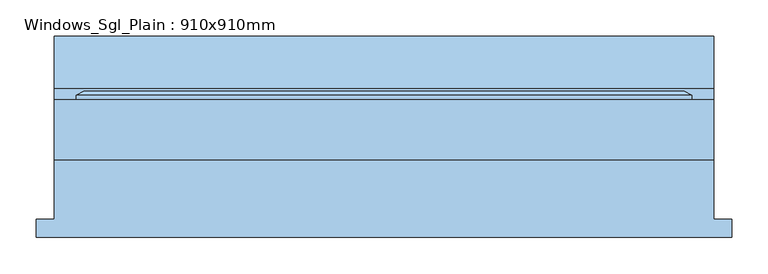
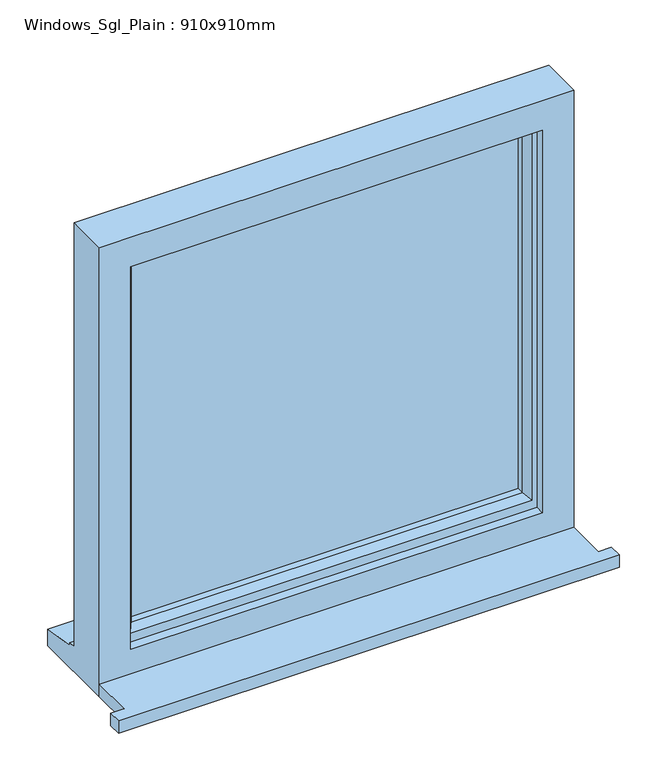
"""IFC4 building model written with IfcOpenShell, lengths in millimetres: window geometry, Windows_Sgl_Plain : 910x910mm."""

from ifc_helpers import new_model, si_unit, frame, origin, place, context, project, spatial, polyline, outline, extrude, faceted_brep, source, transform, mapped, element, save


def windows_sgl_plain_910x910mm_6bfcc678(model_context):
    return source(origin(), model_context, "Body", "SolidModel", [
        extrude(outline(polyline([(-480.0, -124.0434322), (-480.0, -99.0434322), (-455.0, -99.0434322), (-455.0, -17.0434322), (455.0, -17.0434322), (455.0, -99.0434322), (480.0, -99.0434322), (480.0, -124.0434322), (-480.0, -124.0434322)])), frame((0.0, 0.0, 1200.0), z_axis=(0.0, 0.0, 1.0), x_axis=(1.0, 0.0, 0.0)), (0.0, 0.0, 1.0), 25.0),
        faceted_brep([(-455.0, -17.0434322, 1200.0), (455.0, -17.0434322, 1200.0), (455.0, -17.0434322, 2110.0), (-455.0, -17.0434322, 2110.0), (-395.0, -17.0434322, 2050.0), (395.0, -17.0434322, 2050.0), (395.0, -17.0434322, 1275.0), (-395.0, -17.0434322, 1275.0), (-455.0, 65.9565678, 2110.0), (-455.0, 65.9565678, 1251.0), (-455.0, 80.9565678, 1249.68767), (-455.0, 80.9565678, 1244.7449676), (-455.0, 153.4565678, 1233.8088847), (-455.0, 153.4565678, 1200.0), (455.0, 65.9565678, 2110.0), (455.0, 65.9565678, 1251.0), (-415.0, 65.9565678, 2070.0), (-415.0, 65.9565678, 1263.0), (415.0, 65.9565678, 1263.0), (415.0, 65.9565678, 2070.0), (-415.0, 0.9565678, 2070.0), (-415.0, 0.9565678, 1263.0), (415.0, 0.9565678, 2070.0), (415.0, 0.9565678, 1263.0), (-395.0, 0.9565678, 2050.0), (-395.0, 0.9565678, 1275.0), (395.0, 0.9565678, 1275.0), (395.0, 0.9565678, 2050.0), (455.0, 153.4565678, 1200.0), (455.0, 153.4565678, 1233.8088847), (455.0, 80.9565678, 1244.7449676), (455.0, 80.9565678, 1249.68767)], [[[0, 1, 2, 3], [4, 5, 6, 7]], [[0, 3, 8, 9, 10, 11, 12, 13]], [[9, 8, 14, 15], [16, 17, 18, 19]], [[17, 16, 20, 21]], [[20, 22, 23, 21], [24, 25, 26, 27]], [[24, 4, 7, 25]], [[3, 2, 14, 8]], [[16, 19, 22, 20]], [[5, 4, 24, 27]], [[15, 14, 2, 1, 28, 29, 30, 31]], [[19, 18, 23, 22]], [[5, 27, 26, 6]], [[28, 1, 0, 13]], [[29, 28, 13, 12]], [[30, 29, 12, 11]], [[31, 30, 11, 10]], [[15, 31, 10, 9]], [[21, 23, 18, 17]], [[7, 6, 26, 25]]]),
        extrude(outline(polyline([(385.0, 29.9565678), (-385.0, 29.9565678), (-385.0, 53.9565678), (385.0, 53.9565678), (385.0, 29.9565678)])), frame((0.0, 0.0, 1293.0), z_axis=(0.0, 0.0, 1.0), x_axis=(1.0, 0.0, 0.0)), (0.0, 0.0, 1.0), 747.0),
        faceted_brep([(-425.0, 65.9565678, 2080.0), (-425.0, 71.7300705, 2080.0), (-425.0, 71.7300705, 1253.0), (-425.0, 65.9565678, 1253.0), (-415.0, 0.9565678, 2070.0), (-415.0, 65.9565678, 2070.0), (-415.0, 65.9565678, 1263.0), (-415.0, 0.9565678, 1263.0), (-375.0, 15.4494677, 2030.0), (-385.1480377, 0.9565678, 2040.1480377), (-385.1480377, 0.9565678, 1292.8519623), (-375.0, 15.4494677, 1303.0), (-375.0, 29.9565678, 2030.0), (-375.0, 29.9565678, 1303.0), (-385.0, 53.9565678, 2040.0), (-385.0, 29.9565678, 2040.0), (-385.0, 29.9565678, 1293.0), (-385.0, 53.9565678, 1293.0), (-375.0, 71.7300705, 2030.0), (-375.0, 53.9565678, 2030.0), (-375.0, 53.9565678, 1303.0), (-375.0, 71.7300705, 1303.0), (-392.4457548, 77.5035732, 2047.4457548), (-392.4457548, 77.5035732, 1285.5542452), (-414.2153903, 77.5035732, 2069.2153903), (-414.2153903, 77.5035732, 1263.7846097), (425.0, 71.7300705, 1253.0), (425.0, 65.9565678, 1253.0), (415.0, 65.9565678, 1263.0), (415.0, 0.9565678, 1263.0), (385.1480377, 0.9565678, 1292.8519623), (375.0, 15.4494677, 1303.0), (375.0, 29.9565678, 1303.0), (385.0, 29.9565678, 1293.0), (385.0, 53.9565678, 1293.0), (375.0, 53.9565678, 1303.0), (375.0, 71.7300705, 1303.0), (392.4457548, 77.5035732, 1285.5542452), (414.2153903, 77.5035732, 1263.7846097), (425.0, 71.7300705, 2080.0), (425.0, 65.9565678, 2080.0), (415.0, 65.9565678, 2070.0), (415.0, 0.9565678, 2070.0), (385.1480377, 0.9565678, 2040.1480377), (375.0, 15.4494677, 2030.0), (375.0, 29.9565678, 2030.0), (385.0, 29.9565678, 2040.0), (385.0, 53.9565678, 2040.0), (375.0, 53.9565678, 2030.0), (375.0, 71.7300705, 2030.0), (392.4457548, 77.5035732, 2047.4457548), (414.2153903, 77.5035732, 2069.2153903)], [[[0, 1, 2, 3]], [[4, 5, 6, 7]], [[8, 9, 10, 11]], [[12, 8, 11, 13]], [[14, 15, 16, 17]], [[18, 19, 20, 21]], [[22, 18, 21, 23]], [[1, 24, 25, 2]], [[3, 2, 26, 27]], [[7, 6, 28, 29]], [[11, 10, 30, 31]], [[13, 11, 31, 32]], [[17, 16, 33, 34]], [[21, 20, 35, 36]], [[23, 21, 36, 37]], [[2, 25, 38, 26]], [[27, 26, 39, 40]], [[29, 28, 41, 42]], [[31, 30, 43, 44]], [[32, 31, 44, 45]], [[34, 33, 46, 47]], [[36, 35, 48, 49]], [[37, 36, 49, 50]], [[26, 38, 51, 39]], [[40, 39, 1, 0]], [[3, 27, 40, 0], [5, 41, 28, 6]], [[42, 41, 5, 4]], [[7, 29, 42, 4], [9, 43, 30, 10]], [[44, 43, 9, 8]], [[45, 44, 8, 12]], [[15, 46, 33, 16], [13, 32, 45, 12]], [[47, 46, 15, 14]], [[17, 34, 47, 14], [19, 48, 35, 20]], [[49, 48, 19, 18]], [[50, 49, 18, 22]], [[24, 51, 38, 25], [23, 37, 50, 22]], [[39, 51, 24, 1]]]),
    ])


if __name__ == "__main__":
    model = new_model("IFC4")
    model_context = context("Model", 3, world=origin())
    ifc_project = project(units=[si_unit("LENGTHUNIT", "METRE", prefix="MILLI")], contexts=[model_context])
    site = spatial("IfcSite", under=ifc_project)
    building = spatial("IfcBuilding", under=site)
    placement = place(None, origin())
    windows_sgl_plain_910x910mm_shape = windows_sgl_plain_910x910mm_6bfcc678(model_context)
    element("IfcWindow", 1, ObjectType="Windows_Sgl_Plain : 910x910mm", at=placement, inside=building, context=model_context, shape_type="MappedRepresentation", body=[
        mapped(windows_sgl_plain_910x910mm_shape, transform((0.0, 0.0, 0.0), x_axis=(1.0, 0.0, 0.0), y_axis=(0.0, 1.0, 0.0), z_axis=(0.0, 0.0, 1.0))),
    ])
    save(model, "model.ifc")

# Revit data of these elements
# Type "Windows_Sgl_Plain : 910x910mm"
#   Type Mark = "44"
#   Operation = "SinglePanel"
#   Construction Type Id = "SGL"
#   Manufacturer = "Revit"
#   Keynote = "L10"
#   Analytic Construction = "Large single-glazed windows"
#   Wrap Layers (Ext) from Ext = 102.5 mm
#   Wrap Layers (Int) from Ext = 177.5 mm
#   Window Board Projection = 25 mm
#   Window Board Extension = 25 mm
#   Visual Light Transmittance = 0.9
#   Solar Heat Gain Coefficient = 0.86
#   Rough Width = 910 mm
#   Rough Height = 910 mm
#   Height = 910 mm
#   Width = 910 mm
#   Heat Transfer Coefficient (U) = 5.5617 W/(m²·K)
#   Glazing Thickness = 24 mm
#   FrameOffset - External = 50 mm
#   Frame Depth = 65 mm
#   Default Head Height = 2110 mm
#   Cill Depth = 87.5 mm
#   Cavity Closer Width = 50 mm
#   Cavity Closer Offset from Ext = 102.5 mm
#   Cavity Closer Depth = 85 mm
#   Define Thermal Properties by = 1
#   Vis - Cavity Closers = yes
#   Define Thermal Properties by = 1
#   Material Trim = Window Frame
#   Material Glass = Glass
#   Material Frame = Window Frame
#   Wall Closure = (empty or 0)
# Element 1 (IfcWindow, "Windows_Sgl_Plain : 910x910mm")
#   Materials on its faces: "Window Frame", "Glass"
# Materials
#   "Window Frame": colour RGB 249 249 249, transparency 0, Keynote = "L10", Cost = 0
#   "Glass": class "Glass", colour RGB 0 128 192, transparency 0.9, Description = "Soda Lime Glass", Cost = 0
